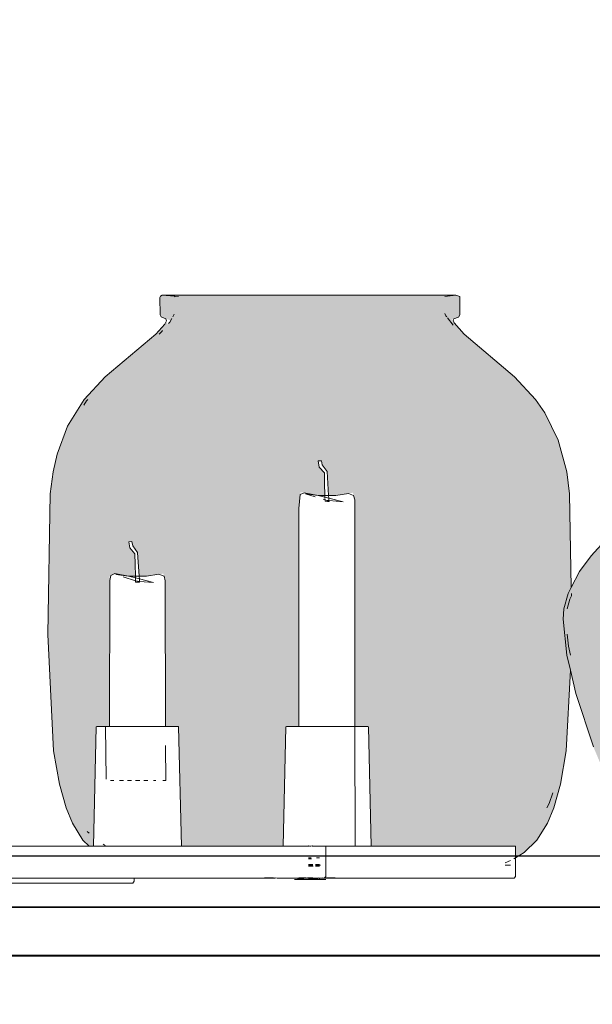
# Model space of a CAD drawing. Units: millimetres. Extents: x 446512 to 447461, y 70395 to 70610.
# Tile 15 of 39: x 446706 to 446712, y 70473 to 70483. Entities that reach past the tile are written whole.
import ezdxf

# ---------------------------------------------------------------- set-up
doc = ezdxf.new("R2010")
doc.units = ezdxf.units.MM
for name, color, linetype, lineweight in [('A-ANNO-DIMS', 2, 'Continuous', 18), ('A-FURN', 7, 'Continuous', 35), ('A-FURN-DECO', 8, 'Continuous', 13), ('A-FURN-PATT', 38, 'Continuous', 13)]:
    doc.layers.add(name, color=color, linetype=linetype, lineweight=lineweight)
doc.styles.get("Standard").update_dxf_attribs({"font": 'arial.ttf'})
doc.dimstyles.get("Standard").update_dxf_attribs({"dimtxt": 0.18, "dimasz": 0.18, "dimexe": 0.18, "dimexo": 0.0625, "dimgap": 0.09, "dimtad": 0, "dimtih": 1, "dimtoh": 1, "dimdec": 4, "dimzin": 0, "dimdsep": 46, "dimtxsty": 'Standard', "dimcen": 0.09, "dimadec": 0, "dimazin": 0, "dimtfac": 1, "dimtdec": 4, "dimtofl": 0, "dimtmove": 0, "dimatfit": 3, "dimfxl": 1, "dimtolj": 1, "dimtzin": 0, "dimarcsym": 0})

# ---------------------------------------------------------------- blocks, each defined once
blk = doc.blocks.new('*D32')
at = {"layer": 'A-ANNO-DIMS', "color": 0, "lineweight": -2, "transparency": 16777216}
for p, q in [((446730.76, 70474.405), (446678.043, 70474.405)), ((446678.223, 70474.225), (446678.223, 70474.075)), ((446678.223, 70473.562), (446678.223, 70473.711)), ((446728.946, 70473.382), (446678.043, 70473.382))]:
    blk.add_line(p, q, dxfattribs=at)
at = {"layer": 'A-ANNO-DIMS', "color": 0, "transparency": 16777216}
for points in [[(446678.193, 70474.225), (446678.253, 70474.225), (446678.223, 70474.405)], [(446678.193, 70473.562), (446678.253, 70473.562), (446678.223, 70473.382)]]:
    blk.add_solid(points, dxfattribs=at)
at = {"layer": 'Defpoints', "color": 0, "transparency": 16777216}
for p in [(446730.822, 70474.405), (446678.223, 70473.382), (446729.008, 70473.382)]:
    blk.add_point(p, dxfattribs=at)
at = {"layer": 'A-ANNO-DIMS', "color": 0, "transparency": 16777216, "insert": (446678.223, 70473.893), "char_height": 0.18, "attachment_point": 5}
blk.add_mtext('\\A1;1.02', dxfattribs=at)

msp = doc.modelspace()

# ---------------------------------------------------------------- hatches: boundary and pattern name
at = {"layer": 'A-FURN-PATT'}
h = msp.add_hatch(color=256, dxfattribs=at)
h.dxf.hatch_style = 1
h.paths.add_polyline_path([(446703.5722, 70477.5476), (446703.5295, 70477.5904), (446703.508, 70477.5904), (446703.383, 70477.6041), (446703.3062, 70477.6039), (446702.8621, 70477.6193), (446702.7177, 70477.6193), (446702.6174, 70477.6163), (446702.576, 70477.615), (446702.5757, 70477.6192), (446702.3373, 70477.6192), (446701.7238, 70477.5898), (446701.6039, 70477.5792), (446701.5612, 70477.5357), (446701.547, 70474.1653), (446703.5225, 70474.1653), (446703.5865, 70474.1653), (446703.5861, 70474.2632), (446703.5852, 70474.4594)])
h.paths.add_polyline_path([(446715.9764, 70475.5286), (446716.1565, 70476.0766), (446716.2492, 70476.4728), (446716.2873, 70476.8422), (446716.2666, 70477.0104), (446716.236, 70477.1061), (446716.1173, 70477.332), (446715.9979, 70477.4937), (446715.8249, 70477.6853), (446715.558, 70477.9316), (446715.2321, 70478.1882), (446714.7182, 70478.5467), (446714.5954, 70478.6535), (446714.3996, 70478.8999), (446714.3461, 70479.0185), (446714.3253, 70479.1028), (446714.3286, 70480.1095), (446714.368, 70480.1364), (446714.3744, 70480.152), (446714.3709, 70480.1808), (446714.3551, 70480.2131), (446714.3271, 70480.2359), (446714.3039, 70480.2478), (446714.2782, 70480.2478), (446714.259, 70480.2458), (446714.2432, 70480.2391), (446714.2375, 70480.2284), (446714.2369, 70480.2218), (446714.2301, 70480.2478), (446713.8255, 70480.2478), (446713.8277, 70480.2375), (446713.8104, 70480.2458), (446713.7912, 70480.2478), (446713.7655, 70480.2478), (446713.738, 70480.2359), (446713.7079, 70480.2028), (446713.6947, 70480.1567), (446713.6986, 70480.1448), (446713.717, 70480.1274), (446713.7341, 70480.1112), (446713.7407, 70480.1049), (446713.7473, 70479.1348), (446713.7233, 70479.0185), (446713.6698, 70478.8999), (446713.5684, 70478.7546), (446713.4739, 70478.6535), (446713.3511, 70478.5467), (446712.8373, 70478.1882), (446712.5114, 70477.9316), (446712.4629, 70477.8868), (446712.2445, 70477.6853), (446712.0714, 70477.4937), (446711.9521, 70477.332), (446711.866, 70477.1682), (446711.8333, 70477.1061), (446711.7899, 70476.9473), (446711.7821, 70476.8422), (446711.8202, 70476.4728), (446711.8563, 70476.3184), (446711.9128, 70476.0766), (446712.093, 70475.5286), (446712.2916, 70475.0627), (446712.4529, 70474.7607), (446712.5622, 70474.5947), (446712.6434, 70474.4935), (446712.7522, 70474.3925), (446712.8451, 70474.3334), (446713.0597, 70474.2483), (446713.2189, 70474.2124), (446713.4296, 70474.1861), (446713.8128, 70474.1834), (446713.5915, 70474.1683), (446714.5392, 70474.1683), (446714.4414, 70474.1779), (446714.1836, 70474.1834), (446714.6098, 70474.1861), (446714.8353, 70474.2124), (446714.9266, 70474.2312), (446715.0097, 70474.2483), (446715.2243, 70474.3334), (446715.3172, 70474.3925), (446715.3727, 70474.4388), (446715.5072, 70474.5947), (446715.6164, 70474.7607), (446715.7778, 70475.0627)])
h.paths.add_polyline_path([(446719.9646, 70475.8685), (446719.9469, 70476.8426), (446719.9277, 70476.9944), (446719.8688, 70477.2155), (446719.7757, 70477.4048), (446719.7115, 70477.4967), (446719.566, 70477.6531), (446719.2165, 70477.9493), (446719.1289, 70478.0481), (446719.1777, 70478.067), (446719.1866, 70478.0815), (446719.1867, 70478.209), (446719.1598, 70478.218), (446719.1369, 70478.2173), (446719.1374, 70478.2174), (446719.0341, 70478.2174), (446718.8666, 70478.218), (446718.6447, 70478.218), (446718.418, 70478.2174), (446718.1448, 70478.2174), (446717.8911, 70478.218), (446717.8873, 70478.218), (446717.6401, 70478.2174), (446717.4215, 70478.2174), (446717.2754, 70478.218), (446717.1987, 70478.218), (446717.2097, 70478.2113), (446717.1243, 70478.2174), (446717.1135, 70478.2124), (446717.1091, 70478.2029), (446717.1111, 70478.0815), (446717.1185, 70478.0683), (446717.1615, 70478.0517), (446717.1433, 70478.0167), (446717.0812, 70477.9493), (446716.7317, 70477.6531), (446716.5862, 70477.4967), (446716.47, 70477.311), (446716.3975, 70477.1183), (446716.37, 70476.9944), (446716.3508, 70476.8426), (446716.3331, 70475.8685), (446716.374, 70475.0624), (446716.4146, 70474.8322), (446716.4608, 70474.6687), (446716.5046, 70474.5619), (446716.5765, 70474.4449), (446716.6659, 70474.36), (446716.7457, 70474.3103), (446716.8351, 70474.2702), (446717.0729, 70474.2085), (446717.2886, 70474.1864), (446717.3803, 70474.1864), (446717.4428, 70474.1846), (446717.4556, 70474.1862), (446718.0146, 70474.1842), (446718.1072, 70474.1795), (446718.1371, 70474.1802), (446718.1473, 70474.1804), (446718.1566, 70474.1797), (446718.1569, 70474.1797), (446718.1592, 70474.1795), (446718.303, 70474.1842), (446719.0393, 70474.1865), (446719.2248, 70474.2085), (446719.365, 70474.2387), (446719.4626, 70474.2702), (446719.552, 70474.3103), (446719.6318, 70474.36), (446719.7212, 70474.4449), (446719.7931, 70474.5619), (446719.8369, 70474.6687), (446719.8831, 70474.8322), (446719.9155, 70475.0156), (446719.9237, 70475.0624)])
h.paths.add_polyline_path([(446718.18, 70474.3158), (446717.2692, 70474.3158), (446717.2092, 70474.3107), (446717.3763, 70474.3107)], flags=16)
h.paths.add_polyline_path([(446717.572, 70474.3384), (446717.5676, 70474.3381), (446717.5691, 70474.3381)], flags=16)
h.paths.add_polyline_path([(446722.3965, 70475.7383), (446722.4453, 70475.7383), (446722.4564, 70475.7383), (446722.4729, 70475.7383), (446722.4785, 70475.7384), (446722.4797, 70475.7383), (446722.4831, 70475.7383), (446722.4841, 70475.7384), (446722.5211, 70475.7384), (446722.4906, 70475.7381), (446722.4906, 70475.7384), (446722.4864, 70475.7383), (446722.4853, 70475.7383), (446722.4831, 70475.7383), (446722.4819, 70475.7383), (446722.4797, 70475.7383), (446722.4618, 70475.7383), (446722.4401, 70475.7383), (446722.4015, 70475.7383), (446722.3964, 70475.7341), (446722.3682, 70474.5084), (446722.5299, 70474.5084), (446723.2721, 70474.5084), (446723.2439, 70475.7341), (446723.2391, 70475.7383), (446723.2067, 70475.7383), (446723.1904, 70475.7383), (446723.1824, 70475.7383), (446723.1499, 70475.7382), (446723.1499, 70475.7384), (446723.1407, 70475.7384), (446723.1819, 70475.7384), (446723.1732, 70475.7384), (446723.1824, 70475.7383), (446723.1957, 70475.7383), (446723.1982, 70475.7383), (446723.2002, 70475.7383), (446723.2067, 70475.7383), (446723.2439, 70475.7383), (446723.2721, 70474.5084), (446724.6768, 70474.5084), (446724.7369, 70474.5652), (446724.8426, 70474.7369), (446724.9068, 70474.8938), (446724.9747, 70475.1338), (446725.0344, 70475.4718), (446725.0943, 70476.6554), (446725.0683, 70478.0856), (446725.0402, 70478.3085), (446724.9998, 70478.4903), (446724.9537, 70478.6331), (446724.8934, 70478.7733), (446724.817, 70478.911), (446724.7228, 70479.046), (446724.5091, 70479.2756), (446724.1522, 70479.5853), (446723.9922, 70479.7544), (446723.8721, 70479.9071), (446723.7862, 70480.0401), (446723.6778, 70480.2901), (446723.6684, 70480.351), (446723.714, 70480.381), (446723.7245, 70480.398), (446723.7213, 70480.4391), (446723.7096, 70480.4663), (446723.6751, 70480.5056), (446723.6405, 70480.5215), (446723.5985, 70480.5218), (446723.5958, 70480.5218), (446722.1196, 70480.5215), (446721.2867, 70480.5218), (446721.2939, 70480.516), (446721.2184, 70480.5218), (446721.1844, 70480.5072), (446721.155, 70480.479), (446721.1354, 70480.4391), (446721.1312, 70480.4035), (446721.1408, 70480.3826), (446721.1891, 70480.3558), (446721.179, 70480.2901), (446721.0706, 70480.0401), (446720.9847, 70479.9071), (446720.8645, 70479.7544), (446720.7046, 70479.5853), (446720.3925, 70479.3145), (446720.3476, 70479.2756), (446720.248, 70479.1783), (446720.134, 70479.046), (446720.0397, 70478.911), (446719.9634, 70478.7733), (446719.9031, 70478.6331), (446719.857, 70478.4903), (446719.8165, 70478.3085), (446719.7884, 70478.0856), (446719.7757, 70477.4048), (446719.8688, 70477.2155), (446719.9277, 70476.9944), (446719.9469, 70476.8426), (446719.9646, 70475.8685), (446719.9237, 70475.0624), (446719.9155, 70475.0156), (446719.9499, 70474.8938), (446720.064, 70474.6452), (446720.1198, 70474.5652), (446720.1819, 70474.4977), (446720.2884, 70474.4145), (446720.3682, 70474.3675), (446720.4995, 70474.3087), (446720.6428, 70474.2625), (446720.8486, 70474.2181), (446720.8834, 70474.214), (446720.8836, 70474.3337), (446720.8838, 70474.5084), (446722.3682, 70474.5084)])
h.paths.add_polyline_path([(446722.5299, 70477.9863), (446722.5458, 70478.1272), (446722.5844, 70478.1453), (446722.7245, 70478.1193), (446722.7937, 70478.1192), (446722.7905, 70478.2404), (446722.7882, 70478.3461), (446722.7354, 70478.4044), (446722.7276, 70478.4661), (446722.759, 70478.4678), (446722.7662, 70478.4254), (446722.8155, 70478.3594), (446722.8317, 70478.1191), (446722.9042, 70478.119), (446723.0314, 70478.1383), (446723.0829, 70478.1185), (446723.0949, 70478.0727), (446723.0974, 70475.7384), (446723.1135, 70475.7383), (446723.104, 70475.7384), (446723.1025, 70475.7384), (446723.0987, 70475.7384), (446723.0974, 70475.7383), (446723.0719, 70475.7383), (446723.018, 70475.7384), (446723.0095, 70475.7382), (446722.9885, 70475.7384), (446722.9576, 70475.7383), (446722.9328, 70475.7384), (446722.9244, 70475.7383), (446722.8841, 70475.7383), (446722.8055, 70475.7384), (446722.802, 70475.7383), (446722.7415, 70475.7384), (446722.7206, 70475.7383), (446722.7104, 70475.7384), (446722.6518, 70475.7384), (446722.6431, 70475.7383), (446722.6067, 70475.7383), (446722.5537, 70475.7384), (446722.5299, 70475.7383)], flags=16)
h.paths.add_polyline_path([(446722.7937, 70478.1192), (446722.8317, 70478.1191), (446722.8336, 70478.0906), (446722.8358, 70478.0578), (446722.7952, 70478.0599), (446722.7946, 70478.0859)], flags=0)
h.paths.add_polyline_path([(446723.5789, 70480.5193), (446723.5569, 70480.5185), (446723.5487, 70480.509)], flags=16)
h = msp.add_hatch(color=256, dxfattribs=at)
h.dxf.hatch_style = 1
h.paths.add_polyline_path([(446709.2643, 70478.4697), (446709.2963, 70478.4714), (446709.3037, 70478.4281), (446709.354, 70478.3607), (446709.3705, 70478.1151), (446709.4446, 70478.1153), (446709.6201, 70478.1418), (446709.6393, 70478.068), (446709.641, 70475.7384), (446709.6528, 70475.7384), (446709.6602, 70475.7385), (446709.7127, 70475.7383), (446709.7148, 70475.7383), (446709.7788, 70475.7385), (446709.8071, 70474.5084), (446711.1855, 70474.5084), (446711.2117, 70474.5083), (446711.22, 70474.5083), (446711.2915, 70474.5089), (446711.2916, 70474.388), (446711.3806, 70474.4434), (446711.5133, 70474.5695), (446711.6201, 70474.7432), (446711.6851, 70474.9019), (446711.7538, 70475.1447), (446711.8141, 70475.4865), (446711.8563, 70476.3184), (446711.8202, 70476.4728), (446711.7821, 70476.8422), (446711.7899, 70476.9473), (446711.8333, 70477.1061), (446711.866, 70477.1682), (446711.8485, 70478.1304), (446711.8201, 70478.3559), (446711.7326, 70478.6842), (446711.5943, 70478.9654), (446711.499, 70479.1019), (446711.2829, 70479.3341), (446710.7638, 70479.774), (446710.6336, 70479.9207), (446710.7062, 70479.9488), (446710.7194, 70479.9704), (446710.7196, 70480.1597), (446710.6824, 70480.1721), (446710.4929, 70480.1721), (446710.2441, 70480.1731), (446709.9146, 70480.1731), (446709.5778, 70480.1721), (446709.1721, 70480.1721), (446708.7954, 70480.1731), (446708.7897, 70480.1731), (446708.4226, 70480.1721), (446708.098, 70480.1721), (446707.8809, 70480.1731), (446707.7178, 70480.1731), (446707.6454, 70480.167), (446707.6405, 70480.1648), (446707.634, 70480.1507), (446707.6369, 70479.9704), (446707.648, 70479.9507), (446707.7452, 70479.9132), (446707.7358, 70479.8967), (446707.7145, 70479.8717), (446707.707, 70479.8983), (446707.5926, 70479.774), (446707.0735, 70479.3341), (446706.8574, 70479.1019), (446706.6848, 70478.8261), (446706.5772, 70478.5398), (446706.5363, 70478.3559), (446706.5078, 70478.1304), (446706.4816, 70476.6838), (446706.5422, 70475.4865), (446706.6026, 70475.1447), (446706.6712, 70474.9019), (446706.7362, 70474.7432), (446706.843, 70474.5695), (446706.9074, 70474.5084), (446706.9519, 70474.5084), (446706.9802, 70475.7383), (446707.0357, 70475.7383), (446707.1156, 70475.7386), (446707.1186, 70477.2864), (446707.1701, 70477.3105), (446707.3128, 70477.284), (446707.3833, 70477.2839), (446707.38, 70477.4074), (446707.3777, 70477.5151), (446707.324, 70477.5745), (446707.316, 70477.6374), (446707.3479, 70477.6391), (446707.3553, 70477.5959), (446707.4056, 70477.5287), (446707.422, 70477.2838), (446707.496, 70477.2837), (446707.6711, 70477.3102), (446707.6902, 70477.2365), (446707.6932, 70475.7383), (446707.7162, 70475.7383), (446707.734, 70475.7385), (446707.7819, 70475.7383), (446707.8276, 70475.7383), (446707.8558, 70474.5084), (446708.9032, 70474.5084), (446708.9314, 70475.7383), (446708.9874, 70475.7383), (446709.0624, 70475.7388), (446709.0624, 70477.9798), (446709.0815, 70478.1491), (446709.2611, 70478.1148), (446709.3317, 70478.115), (446709.3284, 70478.2392), (446709.3261, 70478.3472), (446709.2722, 70478.4067)])

# ---------------------------------------------------------------- linework, layer by layer
at = {"layer": 'A-FURN'}
msp.add_line((446686.5728, 70473.3815), (446746.5728, 70473.3815), dxfattribs=at)
for points in [[(446686.5728, 70493.3815), (446729.0084, 70493.3815), (446729.0084, 70473.3815), (446686.5728, 70473.3815)], [(446687.0728, 70492.8815), (446728.5084, 70492.8815), (446728.5084, 70473.8815), (446687.0728, 70473.8815)], [(446699.4288, 70473.3815), (446746.5728, 70473.3815), (446746.5728, 70453.3815), (446699.4288, 70453.3815)]]:
    msp.add_lwpolyline(points, close=True, dxfattribs=at)
at = {"layer": 'A-FURN-DECO'}
for p, q in [((446707.6405, 70480.1648), (446707.634, 70480.1507)), ((446707.6369, 70479.9704), (446707.634, 70480.1507)), ((446707.6566, 70480.1721), (446707.6405, 70480.1648)), ((446707.7069, 70480.1721), (446707.6566, 70480.1721)), ((446707.6566, 70480.1721), (446707.7834, 70480.1631)), ((446707.7178, 70480.1731), (446707.7069, 70480.1721)), ((446707.7178, 70480.1731), (446707.8809, 70480.1731)), ((446707.7834, 70480.1631), (446707.7847, 70480.1623)), ((446707.7847, 70480.1623), (446707.7913, 70480.1583)), ((446707.7847, 70480.1623), (446707.8258, 70480.1592)), ((446707.8258, 70480.1592), (446707.8278, 70480.1593)), ((446708.098, 70480.1721), (446707.8809, 70480.1731)), ((446708.098, 70480.1721), (446708.4226, 70480.1721)), ((446708.4226, 70480.1721), (446708.7838, 70480.1731)), ((446708.7838, 70480.1731), (446708.7897, 70480.1731)), ((446708.7897, 70480.1731), (446708.7954, 70480.1731)), ((446708.7954, 70480.1731), (446709.1721, 70480.1721)), ((446709.5778, 70480.1721), (446709.1721, 70480.1721)), ((446709.9237, 70480.1731), (446709.5778, 70480.1721)), ((446709.9402, 70480.1731), (446709.9237, 70480.1731)), ((446709.9402, 70480.1731), (446710.2441, 70480.1731)), ((446710.4929, 70480.1721), (446710.2441, 70480.1731)), ((446710.4929, 70480.1721), (446710.6494, 70480.1721)), ((446710.5641, 70480.1584), (446710.6796, 70480.1731)), ((446710.6494, 70480.1721), (446710.6796, 70480.1731)), ((446710.6796, 70480.1731), (446710.7196, 70480.1597)), ((446710.7196, 70480.1597), (446710.7194, 70479.9704)), ((446707.6369, 70479.9704), (446707.648, 70479.9507)), ((446707.648, 70479.9507), (446707.6976, 70479.9316)), ((446707.6976, 70479.9316), (446707.7036, 70479.9104)), ((446707.7358, 70479.8967), (446707.7573, 70479.9346)), ((446707.7667, 70479.9512), (446707.7814, 70479.977)), ((446710.5759, 70479.9621), (446710.5643, 70479.9866)), ((446710.5855, 70479.9498), (446710.5759, 70479.9621)), ((446710.6513, 70479.8659), (446710.5925, 70479.9409)), ((446710.6566, 70479.9296), (446710.652, 70479.9183)), ((446710.7062, 70479.9488), (446710.6566, 70479.9296)), ((446710.7194, 70479.9704), (446710.7062, 70479.9488)), ((446707.6848, 70479.8741), (446707.5926, 70479.774)), ((446707.7036, 70479.9104), (446707.6848, 70479.8741)), ((446707.7358, 70479.8967), (446707.7245, 70479.8834)), ((446710.652, 70479.9183), (446710.6622, 70479.8885)), ((446710.6622, 70479.8885), (446710.7638, 70479.774)), ((446707.5926, 70479.774), (446707.0735, 70479.3341)), ((446707.6262, 70479.774), (446707.6539, 70479.8005)), ((446707.6609, 70479.8088), (446707.6539, 70479.8005)), ((446710.7638, 70479.774), (446711.2829, 70479.3341)), ((446707.0735, 70479.3341), (446706.8574, 70479.1019)), ((446711.2829, 70479.3341), (446711.499, 70479.1019)), ((446706.8574, 70479.1019), (446706.6848, 70478.8261)), ((446706.8529, 70479.0442), (446706.8812, 70479.086)), ((446706.8812, 70479.086), (446706.8945, 70479.1019)), ((446711.499, 70479.1019), (446711.5943, 70478.9654)), ((446711.5943, 70478.9654), (446711.7326, 70478.6842)), ((446706.6848, 70478.8261), (446706.5772, 70478.5398)), ((446711.7326, 70478.6842), (446711.8201, 70478.3559)), ((446706.5772, 70478.5398), (446706.5363, 70478.3559)), ((446709.2963, 70478.4714), (446709.2643, 70478.4697)), ((446709.2722, 70478.4067), (446709.2643, 70478.4697)), ((446709.3261, 70478.3472), (446709.2722, 70478.4067)), ((446709.3037, 70478.4281), (446709.2963, 70478.4714)), ((446709.354, 70478.3607), (446709.3037, 70478.4281)), ((446706.5363, 70478.3559), (446706.5078, 70478.1304)), ((446709.3284, 70478.2392), (446709.3261, 70478.3472)), ((446709.354, 70478.3607), (446709.3705, 70478.1151)), ((446711.8201, 70478.3559), (446711.8485, 70478.1304)), ((446709.3317, 70478.115), (446709.3284, 70478.2392)), ((446706.5078, 70478.1304), (446706.4816, 70476.6838)), ((446709.0624, 70477.9798), (446709.0786, 70478.1236)), ((446709.1181, 70478.1421), (446709.0786, 70478.1236)), ((446709.1181, 70478.1421), (446709.2611, 70478.1148)), ((446709.1313, 70478.1322), (446709.2611, 70478.1148)), ((446709.2325, 70478.1004), (446709.1313, 70478.1322)), ((446709.3317, 70478.115), (446709.2611, 70478.1148)), ((446709.3322, 70478.0966), (446709.2611, 70478.1148)), ((446709.3705, 70478.1151), (446709.3317, 70478.115)), ((446709.3322, 70478.0966), (446709.3317, 70478.115)), ((446709.3324, 70478.0904), (446709.3322, 70478.0966)), ((446709.3725, 70478.0863), (446709.3322, 70478.0966)), ((446709.4446, 70478.1153), (446709.3705, 70478.1151)), ((446709.3705, 70478.1151), (446709.3725, 70478.0863)), ((446709.5744, 70478.1349), (446709.4446, 70478.1153)), ((446709.6271, 70478.1148), (446709.5744, 70478.1349)), ((446709.6393, 70478.068), (446709.6271, 70478.1148)), ((446711.8485, 70478.1304), (446711.866, 70477.1682)), ((446709.333, 70478.069), (446709.3132, 70478.0752)), ((446709.333, 70478.069), (446709.3326, 70478.0815)), ((446709.3528, 70478.0628), (446709.333, 70478.069)), ((446709.3333, 70478.0549), (446709.333, 70478.069)), ((446709.3589, 70478.0536), (446709.3333, 70478.0549)), ((446709.3742, 70478.061), (446709.3528, 70478.0628)), ((446709.3589, 70478.0536), (446709.3747, 70478.0532)), ((446709.3725, 70478.0863), (446709.3737, 70478.0684)), ((446709.5189, 70478.0488), (446709.3725, 70478.0863)), ((446709.3742, 70478.061), (446709.3747, 70478.0532)), ((446709.5189, 70478.0488), (446709.3742, 70478.061)), ((446709.641, 70475.7383), (446709.6393, 70478.068)), ((446709.0624, 70475.7383), (446709.0624, 70477.9798)), ((446707.3479, 70477.6391), (446707.316, 70477.6374)), ((446707.324, 70477.5745), (446707.316, 70477.6374)), ((446707.3553, 70477.5959), (446707.3479, 70477.6391)), ((446707.4056, 70477.5287), (446707.3553, 70477.5959)), ((446712.0714, 70477.4937), (446712.2445, 70477.6853)), ((446707.3777, 70477.5151), (446707.324, 70477.5745)), ((446707.38, 70477.4074), (446707.3777, 70477.5151)), ((446707.4056, 70477.5287), (446707.422, 70477.2838)), ((446712.0714, 70477.4937), (446711.9521, 70477.332)), ((446707.3833, 70477.2839), (446707.38, 70477.4074)), ((446707.1186, 70477.2402), (446707.1307, 70477.292)), ((446707.1307, 70477.292), (446707.1701, 70477.3105)), ((446707.1701, 70477.3105), (446707.3128, 70477.284)), ((446707.1833, 70477.3006), (446707.3128, 70477.284)), ((446707.496, 70477.2837), (446707.6255, 70477.3033)), ((446707.6781, 70477.2832), (446707.6255, 70477.3033)), ((446711.9521, 70477.332), (446711.866, 70477.1682)), ((446707.1156, 70475.7383), (446707.1186, 70477.2402)), ((446707.2576, 70477.2773), (446707.3845, 70477.2375)), ((446707.3128, 70477.284), (446707.3833, 70477.2839)), ((446707.3128, 70477.284), (446707.3838, 70477.2656)), ((446707.3833, 70477.2839), (446707.422, 70477.2838)), ((446707.3838, 70477.2656), (446707.3833, 70477.2839)), ((446707.3838, 70477.2656), (446707.424, 70477.2552)), ((446707.3845, 70477.2375), (446707.3838, 70477.2656)), ((446707.3845, 70477.2375), (446707.4044, 70477.2313)), ((446707.3849, 70477.2235), (446707.3845, 70477.2375)), ((446707.4104, 70477.2221), (446707.3849, 70477.2235)), ((446707.4257, 70477.2295), (446707.4044, 70477.2313)), ((446707.4104, 70477.2221), (446707.4262, 70477.2217)), ((446707.422, 70477.2838), (446707.496, 70477.2837)), ((446707.422, 70477.2838), (446707.424, 70477.2552)), ((446707.424, 70477.2552), (446707.5701, 70477.2174)), ((446707.424, 70477.2552), (446707.4257, 70477.2295)), ((446707.5701, 70477.2174), (446707.4257, 70477.2295)), ((446707.4257, 70477.2295), (446707.4262, 70477.2217)), ((446707.6902, 70477.2365), (446707.6781, 70477.2832)), ((446707.6902, 70477.2365), (446707.6932, 70475.7383)), ((446711.7899, 70476.9473), (446711.8333, 70477.1061)), ((446711.866, 70477.1682), (446711.8333, 70477.1061)), ((446711.8671, 70477.1061), (446711.869, 70477.0887)), ((446711.869, 70477.0887), (446711.8675, 70477.0855)), ((446711.8675, 70477.0855), (446711.8675, 70477.0832)), ((446711.8249, 70476.9473), (446711.8502, 70477.0483)), ((446711.8675, 70477.0832), (446711.8502, 70477.0483)), ((446711.7821, 70476.8422), (446711.7899, 70476.9473)), ((446711.7821, 70476.8422), (446711.8202, 70476.4728)), ((446706.4816, 70476.6838), (446706.5422, 70475.4865)), ((446711.822, 70476.687), (446711.8374, 70476.5647)), ((446711.8374, 70476.5647), (446711.8584, 70476.4728)), ((446711.8563, 70476.3184), (446711.8202, 70476.4728)), ((446711.8563, 70476.3184), (446711.8141, 70475.4865)), ((446711.9128, 70476.0766), (446711.8563, 70476.3184)), ((446712.093, 70475.5286), (446711.9128, 70476.0766)), ((446706.9519, 70474.5084), (446706.9801, 70475.7341)), ((446706.9801, 70475.7341), (446706.9852, 70475.7383)), ((446706.9852, 70475.7383), (446707.0357, 70475.7383)), ((446707.0357, 70475.7383), (446707.0401, 70475.7383)), ((446707.0401, 70475.7383), (446707.043, 70475.7383)), ((446707.043, 70475.7383), (446707.0455, 70475.7383)), ((446707.0455, 70475.7383), (446707.0467, 70475.7383)), ((446707.0467, 70475.7383), (446707.0534, 70475.7384)), ((446707.0534, 70475.7384), (446707.0657, 70475.7383)), ((446707.0657, 70475.7383), (446707.0676, 70475.7384)), ((446707.0676, 70475.7384), (446707.0703, 70475.7384)), ((446707.0703, 70475.7384), (446707.0743, 70475.7384)), ((446707.0743, 70475.7384), (446707.0822, 70475.1981)), ((446707.0743, 70475.7384), (446707.0841, 70475.7384)), ((446707.0841, 70475.7384), (446707.0948, 70475.7383)), ((446707.0948, 70475.7383), (446707.1049, 70475.7384)), ((446707.1049, 70475.7384), (446707.1062, 70475.7384)), ((446707.1139, 70475.7383), (446707.1062, 70475.7384)), ((446707.1156, 70475.7383), (446707.1139, 70475.7383)), ((446707.1156, 70475.7341), (446707.1156, 70475.7383)), ((446707.1156, 70475.7383), (446707.1384, 70475.7383)), ((446707.1384, 70475.7383), (446707.1397, 70475.7384)), ((446707.1397, 70475.7384), (446707.1834, 70475.7384)), ((446707.1904, 70475.7383), (446707.1834, 70475.7384)), ((446707.1904, 70475.7383), (446707.2085, 70475.7384)), ((446707.3043, 70475.7383), (446707.2085, 70475.7384)), ((446707.3043, 70475.7383), (446707.3252, 70475.7384)), ((446707.3857, 70475.7383), (446707.3252, 70475.7384)), ((446707.3857, 70475.7383), (446707.3892, 70475.7384)), ((446707.3892, 70475.7384), (446707.4216, 70475.7384)), ((446707.4269, 70475.7383), (446707.4216, 70475.7384)), ((446707.4269, 70475.7383), (446707.4856, 70475.7384)), ((446707.5081, 70475.7383), (446707.4856, 70475.7384)), ((446707.6017, 70475.7384), (446707.5081, 70475.7383)), ((446707.6017, 70475.7384), (446707.6215, 70475.7383)), ((446707.6215, 70475.7383), (446707.6267, 70475.7384)), ((446707.6267, 70475.7384), (446707.6703, 70475.7383)), ((446707.6703, 70475.7383), (446707.6932, 70475.7383)), ((446707.6932, 70475.7383), (446707.6932, 70475.7341)), ((446707.7162, 70475.7383), (446707.6932, 70475.7383)), ((446707.7162, 70475.7383), (446707.7187, 70475.7383)), ((446707.7187, 70475.7383), (446707.7207, 70475.7383)), ((446707.7207, 70475.7383), (446707.7301, 70475.7384)), ((446707.7336, 70475.7384), (446707.7301, 70475.7384)), ((446707.7336, 70475.7384), (446707.7336, 70475.7341)), ((446707.7623, 70475.7383), (446707.7336, 70475.7384)), ((446707.7623, 70475.7383), (446707.7648, 70475.7383)), ((446707.7705, 70475.7383), (446707.7648, 70475.7383)), ((446707.7819, 70475.7383), (446707.7705, 70475.7383)), ((446707.7819, 70475.7383), (446707.8228, 70475.7383)), ((446707.8277, 70475.7341), (446707.8228, 70475.7383)), ((446707.8558, 70474.5084), (446707.8277, 70475.7341)), ((446708.9032, 70474.5084), (446708.9313, 70475.7341)), ((446708.9313, 70475.7341), (446708.9364, 70475.7383)), ((446708.9364, 70475.7383), (446708.9874, 70475.7383)), ((446708.9919, 70475.7383), (446708.9874, 70475.7383)), ((446709.0106, 70475.7383), (446708.9919, 70475.7383)), ((446709.0169, 70475.7383), (446709.0106, 70475.7383)), ((446709.0198, 70475.7383), (446709.0169, 70475.7383)), ((446709.0255, 70475.7384), (446709.0198, 70475.7383)), ((446709.0255, 70475.7384), (446709.0353, 70475.7384)), ((446709.0255, 70475.7384), (446709.0255, 70475.7341)), ((446709.0428, 70475.7383), (446709.0353, 70475.7384)), ((446709.0485, 70475.7384), (446709.0428, 70475.7383)), ((446709.0561, 70475.7384), (446709.0485, 70475.7384)), ((446709.0574, 70475.7384), (446709.0561, 70475.7384)), ((446709.0624, 70475.7383), (446709.0574, 70475.7384)), ((446709.0712, 70475.7384), (446709.0624, 70475.7383)), ((446709.0624, 70475.7341), (446709.0624, 70475.7383)), ((446709.0753, 70475.7383), (446709.0712, 70475.7384)), ((446709.0753, 70475.7383), (446709.081, 70475.7383)), ((446709.081, 70475.7383), (446709.0867, 70475.7383)), ((446709.0867, 70475.7383), (446709.0909, 70475.7384)), ((446709.0909, 70475.7384), (446709.1073, 70475.7383)), ((446709.1073, 70475.7383), (446709.1116, 70475.7384)), ((446709.1116, 70475.7384), (446709.1474, 70475.7383)), ((446709.1474, 70475.7383), (446709.1573, 70475.7384)), ((446709.1573, 70475.7384), (446709.1597, 70475.7384)), ((446709.178, 70475.7383), (446709.1597, 70475.7384)), ((446709.178, 70475.7383), (446709.1868, 70475.7384)), ((446709.2053, 70475.7383), (446709.1868, 70475.7384)), ((446709.2053, 70475.7383), (446709.2454, 70475.7384)), ((446709.2556, 70475.7383), (446709.2454, 70475.7384)), ((446709.2556, 70475.7383), (446709.3082, 70475.7384)), ((446709.337, 70475.7383), (446709.3082, 70475.7384)), ((446709.337, 70475.7383), (446709.3729, 70475.7384)), ((446709.419, 70475.7383), (446709.3729, 70475.7384)), ((446709.419, 70475.7383), (446709.4368, 70475.7384)), ((446709.4368, 70475.7384), (446709.4976, 70475.7384)), ((446709.4991, 70475.7383), (446709.4976, 70475.7384)), ((446709.4991, 70475.7383), (446709.5235, 70475.7384)), ((446709.5235, 70475.7384), (446709.5444, 70475.7383)), ((446709.553, 70475.7384), (446709.5444, 70475.7383)), ((446709.5571, 70475.7383), (446709.553, 70475.7384)), ((446709.5571, 70475.7383), (446709.5728, 70475.7383)), ((446709.5728, 70475.7383), (446709.6007, 70475.7384)), ((446709.6331, 70475.7383), (446709.6007, 70475.7384)), ((446709.635, 70475.7383), (446709.6331, 70475.7383)), ((446709.6385, 70475.7383), (446709.635, 70475.7383)), ((446709.641, 70475.7383), (446709.6385, 70475.7383)), ((446709.642, 70474.5084), (446709.641, 70475.7383)), ((446709.6437, 70475.7383), (446709.641, 70475.7383)), ((446709.6462, 70475.7384), (446709.6437, 70475.7383)), ((446709.6476, 70475.7383), (446709.6462, 70475.7384)), ((446709.6512, 70475.7383), (446709.6476, 70475.7383)), ((446709.6528, 70475.7384), (446709.6512, 70475.7383)), ((446709.6551, 70475.7383), (446709.6528, 70475.7384)), ((446709.6567, 70475.7384), (446709.6551, 70475.7383)), ((446709.6642, 70475.7383), (446709.6567, 70475.7384)), ((446709.6664, 70475.7384), (446709.6642, 70475.7383)), ((446709.6664, 70475.7384), (446709.6687, 70475.7383)), ((446709.6687, 70475.7383), (446709.6814, 70475.7384)), ((446709.6848, 70475.7384), (446709.6814, 70475.7384)), ((446709.6848, 70475.7384), (446709.6848, 70475.7341)), ((446709.6933, 70475.7383), (446709.6848, 70475.7384)), ((446709.6957, 70475.7383), (446709.6933, 70475.7383)), ((446709.6993, 70475.7384), (446709.6957, 70475.7383)), ((446709.7015, 70475.7384), (446709.6993, 70475.7384)), ((446709.7135, 70475.7383), (446709.7015, 70475.7384)), ((446709.7248, 70475.7383), (446709.7135, 70475.7383)), ((446709.73, 70475.7383), (446709.7248, 70475.7383)), ((446709.73, 70475.7383), (446709.7738, 70475.7383)), ((446709.7789, 70475.7341), (446709.7738, 70475.7383)), ((446709.8071, 70474.5084), (446709.7789, 70475.7341)), ((446706.5422, 70475.4865), (446706.6026, 70475.1447)), ((446707.6936, 70475.5422), (446707.6943, 70475.1831)), ((446711.8141, 70475.4865), (446711.7538, 70475.1447)), ((446707.1264, 70475.1831), (446707.1608, 70475.1831)), ((446707.2592, 70475.1831), (446707.2194, 70475.1831)), ((446707.3423, 70475.1831), (446707.3003, 70475.1831)), ((446707.385, 70475.1831), (446707.4279, 70475.1831)), ((446707.5125, 70475.1831), (446707.4705, 70475.1831)), ((446707.593, 70475.1831), (446707.5701, 70475.1831)), ((446707.6943, 70475.1831), (446707.6662, 70475.1831)), ((446706.6026, 70475.1447), (446706.6712, 70474.9019)), ((446711.7538, 70475.1447), (446711.6851, 70474.9019)), ((446711.6382, 70474.9476), (446711.6746, 70475.0553)), ((446706.6712, 70474.9019), (446706.7362, 70474.7432)), ((446711.6144, 70474.9019), (446711.6382, 70474.9476)), ((446711.6851, 70474.9019), (446711.6201, 70474.7432)), ((446706.7362, 70474.7432), (446706.843, 70474.5695)), ((446706.9062, 70474.6405), (446706.8871, 70474.6584)), ((446711.6201, 70474.7432), (446711.5133, 70474.5695)), ((446706.843, 70474.5695), (446706.9074, 70474.5084)), ((446711.5133, 70474.5695), (446711.3806, 70474.4434)), ((446706.9074, 70474.5084), (446705.8852, 70474.5084)), ((446706.9074, 70474.5084), (446706.9519, 70474.5084)), ((446707.8558, 70474.5084), (446706.9519, 70474.5084)), ((446707.0707, 70474.5156), (446707.0502, 70474.5266)), ((446708.9032, 70474.5084), (446707.8558, 70474.5084)), ((446709.1642, 70474.5084), (446708.9032, 70474.5084)), ((446709.1679, 70474.5104), (446709.1642, 70474.5098)), ((446709.1679, 70474.5104), (446709.1642, 70474.5084)), ((446709.1726, 70474.5084), (446709.1679, 70474.5104)), ((446709.1726, 70474.5084), (446709.1879, 70474.5084)), ((446709.1879, 70474.5084), (446709.2008, 70474.5104)), ((446709.2008, 70474.5104), (446709.2053, 70474.5084)), ((446709.2008, 70474.5104), (446709.2053, 70474.5103)), ((446709.2053, 70474.5084), (446709.2342, 70474.5084)), ((446709.2342, 70474.5084), (446709.2605, 70474.5083)), ((446709.2687, 70474.5083), (446709.2605, 70474.5083)), ((446709.2687, 70474.5083), (446709.2772, 70474.5084)), ((446709.3402, 70474.5084), (446709.2772, 70474.5084)), ((446709.3407, 70474.1952), (446709.3402, 70474.5084)), ((446709.3402, 70474.5084), (446709.642, 70474.5084)), ((446709.642, 70474.5084), (446709.8071, 70474.5084)), ((446709.8071, 70474.5084), (446711.1855, 70474.5084)), ((446711.1855, 70474.5084), (446711.2117, 70474.5083)), ((446711.22, 70474.5083), (446711.2117, 70474.5083)), ((446711.2307, 70474.5084), (446711.22, 70474.5083)), ((446711.2307, 70474.5084), (446711.2915, 70474.5084)), ((446711.2916, 70474.388), (446711.2915, 70474.5084)), ((446709.171, 70474.3874), (446709.1632, 70474.3872)), ((446709.1632, 70474.3813), (446709.1921, 70474.3813)), ((446709.1929, 70474.3778), (446709.1632, 70474.3778)), ((446709.1909, 70474.3867), (446709.171, 70474.3874)), ((446709.2472, 70474.3874), (446709.2772, 70474.3874)), ((446711.2393, 70474.3594), (446711.1857, 70474.3354)), ((446711.2916, 70474.388), (446711.2747, 70474.3775)), ((446711.3806, 70474.4434), (446711.2916, 70474.388)), ((446711.2919, 70474.1952), (446711.2916, 70474.388)), ((446709.1633, 70474.3202), (446709.2061, 70474.3202)), ((446709.208, 70474.3119), (446709.1633, 70474.3116)), ((446709.1633, 70474.3031), (446709.21, 70474.3031)), ((446709.2772, 70474.3202), (446709.2345, 70474.3202)), ((446709.2708, 70474.3123), (446709.2345, 70474.312)), ((446709.276, 70474.3031), (446709.2345, 70474.3031)), ((446709.2345, 70474.3031), (446709.2772, 70474.3025)), ((446709.2881, 70474.3123), (446709.2708, 70474.3123)), ((446711.222, 70474.3123), (446711.1858, 70474.3121)), ((446711.2393, 70474.3123), (446711.222, 70474.3123)), ((446705.6724, 70474.1775), (446707.3711, 70474.1775)), ((446707.3712, 70474.1463), (446707.3711, 70474.1775)), ((446707.3711, 70474.1775), (446708.7232, 70474.1775)), ((446708.7091, 70474.179), (446708.7232, 70474.1775)), ((446708.8199, 70474.1805), (446708.7098, 70474.1803)), ((446708.7115, 70474.1832), (446708.8032, 70474.1829)), ((446708.7517, 70474.1777), (446708.7232, 70474.1775)), ((446708.8199, 70474.1805), (446708.7517, 70474.1777)), ((446708.8176, 70474.1775), (446708.7517, 70474.1777)), ((446708.8199, 70474.1805), (446708.8176, 70474.1775)), ((446708.8406, 70474.1775), (446708.8199, 70474.1805)), ((446709.0626, 70474.1776), (446708.8406, 70474.1775)), ((446709.1164, 70474.1753), (446709.02, 70474.1634)), ((446709.02, 70474.1634), (446709.3203, 70474.1634)), ((446709.0898, 70474.1775), (446709.0626, 70474.1776)), ((446709.121, 70474.1823), (446709.0642, 70474.1798)), ((446709.0642, 70474.1798), (446709.0898, 70474.1775)), ((446709.121, 70474.1823), (446709.0651, 70474.1811)), ((446709.0898, 70474.1775), (446709.1095, 70474.1782)), ((446709.0898, 70474.1775), (446709.1164, 70474.1753)), ((446709.1095, 70474.1782), (446709.1229, 70474.1778)), ((446709.1229, 70474.1778), (446709.1164, 70474.1753)), ((446709.1305, 70474.1812), (446709.121, 70474.1823)), ((446709.1309, 70474.1775), (446709.1229, 70474.1778)), ((446709.1344, 70474.1812), (446709.1305, 70474.1812)), ((446709.1354, 70474.1775), (446709.1309, 70474.1775)), ((446709.1344, 70474.1812), (446709.1382, 70474.1803)), ((446709.1448, 70474.1787), (446709.1354, 70474.1775)), ((446709.1485, 70474.1779), (446709.1448, 70474.1787)), ((446709.151, 70474.1788), (446709.1485, 70474.1779)), ((446709.1485, 70474.1779), (446709.1503, 70474.1779)), ((446709.1503, 70474.1779), (446709.1592, 70474.1778)), ((446709.151, 70474.1788), (446709.1592, 70474.1778)), ((446709.2082, 70474.1814), (446709.1529, 70474.1813)), ((446709.1592, 70474.1778), (446709.1615, 70474.1775)), ((446709.1615, 70474.1775), (446709.1646, 70474.1763)), ((446709.1646, 70474.1763), (446709.1667, 70474.1775)), ((446709.1667, 70474.1775), (446709.1703, 70474.1765)), ((446709.1703, 70474.1765), (446709.174, 70474.176)), ((446709.174, 70474.176), (446709.1779, 70474.1766)), ((446709.1779, 70474.1766), (446709.1795, 70474.1753)), ((446709.1795, 70474.1753), (446709.1897, 70474.1756)), ((446709.1897, 70474.1756), (446709.1935, 70474.1753)), ((446709.2082, 70474.1814), (446709.1935, 70474.1753)), ((446709.2092, 70474.1775), (446709.1935, 70474.1753)), ((446709.1935, 70474.1753), (446709.3203, 70474.1634)), ((446709.2082, 70474.1814), (446709.2137, 70474.1797)), ((446709.2092, 70474.1775), (446709.2603, 70474.1775)), ((446709.2603, 70474.1775), (446709.2651, 70474.1815)), ((446709.2651, 70474.1815), (446709.2739, 70474.1775)), ((446709.2778, 70474.1775), (446709.2739, 70474.1775)), ((446709.3043, 70474.1816), (446709.2778, 70474.1775)), ((446709.2778, 70474.1775), (446709.3041, 70474.1775)), ((446709.3071, 70474.1792), (446709.3041, 70474.1775)), ((446709.3091, 70474.1775), (446709.3071, 70474.1792)), ((446709.3091, 70474.1775), (446709.3259, 70474.1775)), ((446709.3417, 70474.1634), (446709.3203, 70474.1634)), ((446709.3254, 70474.1816), (446709.3271, 70474.1818)), ((446709.3279, 70474.1799), (446709.3254, 70474.1816)), ((446709.3256, 70474.1798), (446709.3279, 70474.1799)), ((446709.3259, 70474.1775), (446709.3256, 70474.1798)), ((446709.3259, 70474.1775), (446710.5147, 70474.1775)), ((446709.3271, 70474.1818), (446709.3294, 70474.1816)), ((446709.3294, 70474.1816), (446709.3279, 70474.1799)), ((446709.3294, 70474.1816), (446709.3407, 70474.1952)), ((446709.3294, 70474.1816), (446709.3341, 70474.1818)), ((446709.3353, 70474.1818), (446709.3341, 70474.1818)), ((446709.3411, 70474.1818), (446709.3353, 70474.1818)), ((446709.3432, 70474.1817), (446709.3411, 70474.1818)), ((446709.3449, 70474.1818), (446709.3432, 70474.1817)), ((446709.3432, 70474.1817), (446709.3468, 70474.1817)), ((446709.3468, 70474.1817), (446709.3449, 70474.1818)), ((446709.3468, 70474.1817), (446709.3491, 70474.1817)), ((446709.3534, 70474.1817), (446709.3491, 70474.1817)), ((446709.3534, 70474.1817), (446709.3549, 70474.1818)), ((446709.3575, 70474.1817), (446709.3549, 70474.1818)), ((446709.3589, 70474.1818), (446709.3575, 70474.1817)), ((446709.3575, 70474.1817), (446709.3603, 70474.1817)), ((446709.3617, 70474.1817), (446709.3589, 70474.1818)), ((446709.3603, 70474.1817), (446709.3617, 70474.1817)), ((446709.3632, 70474.1817), (446709.3617, 70474.1817)), ((446709.3658, 70474.1818), (446709.3632, 70474.1817)), ((446709.3683, 70474.1816), (446709.3658, 70474.1818)), ((446709.3683, 70474.1816), (446709.3718, 70474.1818)), ((446709.3683, 70474.1816), (446709.3702, 70474.1816)), ((446709.3702, 70474.1816), (446709.3718, 70474.1818)), ((446709.3718, 70474.1818), (446709.3753, 70474.1813)), ((446709.3753, 70474.1813), (446709.3786, 70474.1815)), ((446709.3786, 70474.1815), (446709.3809, 70474.1816)), ((446709.3831, 70474.1818), (446709.3809, 70474.1816)), ((446709.3849, 70474.1818), (446709.3831, 70474.1818)), ((446709.3849, 70474.1818), (446709.387, 70474.1816)), ((446709.387, 70474.1816), (446709.3896, 70474.1818)), ((446709.3909, 70474.1818), (446709.3896, 70474.1818)), ((446709.3909, 70474.1818), (446709.4072, 70474.1823)), ((446709.4151, 70474.1823), (446709.4072, 70474.1823)), ((446709.4359, 70474.1804), (446709.4151, 70474.1823)), ((446710.5147, 70474.1775), (446710.6597, 70474.1778)), ((446710.6597, 70474.1778), (446710.7689, 70474.1775)), ((446710.7689, 70474.1775), (446710.7851, 70474.1785)), ((446710.7918, 70474.1775), (446710.7851, 70474.1785)), ((446710.9962, 70474.1775), (446710.7918, 70474.1775)), ((446710.9962, 70474.1775), (446711.0107, 70474.1781)), ((446711.012, 70474.1779), (446710.9962, 70474.1775)), ((446711.014, 70474.1778), (446711.012, 70474.1779)), ((446711.014, 70474.1778), (446711.0866, 70474.1775)), ((446711.1001, 70474.1778), (446711.0866, 70474.1775)), ((446711.1001, 70474.1778), (446711.1014, 70474.1778)), ((446711.1014, 70474.1778), (446711.1604, 70474.1775)), ((446711.172, 70474.1776), (446711.1604, 70474.1775)), ((446711.172, 70474.1776), (446711.225, 70474.1776)), ((446711.225, 70474.1776), (446711.2553, 70474.1775)), ((446711.2603, 70474.1775), (446711.2553, 70474.1775)), ((446711.2603, 70474.1775), (446711.2771, 70474.1775)), ((446711.2771, 70474.1775), (446711.2919, 70474.1952)), ((446706.0663, 70474.1286), (446707.3564, 70474.1286)), ((446707.3564, 70474.1286), (446707.3712, 70474.1463))]:
    msp.add_line(p, q, dxfattribs=at)

# ---------------------------------------------------------------- dimensions: what is measured, and where the dimension line sits
at = {"layer": 'A-ANNO-DIMS'}
dim = msp.add_linear_dim(base=(446678.2228, 70473.3815), p1=(446730.8224, 70474.4047), p2=(446729.0084, 70473.3815), angle=90, dimstyle='Standard', override={"dimdec": 2, "dimlfac": 1, "dimrnd": 0, "dimzin": 0, "dimdsep": 46, "dimlunit": 2}, dxfattribs=at)
dim.commit()
dim.dimension.update_dxf_attribs({"geometry": '*D32', "text_midpoint": (446678.2228, 70473.8931)})

doc.saveas('drawing.dxf')
